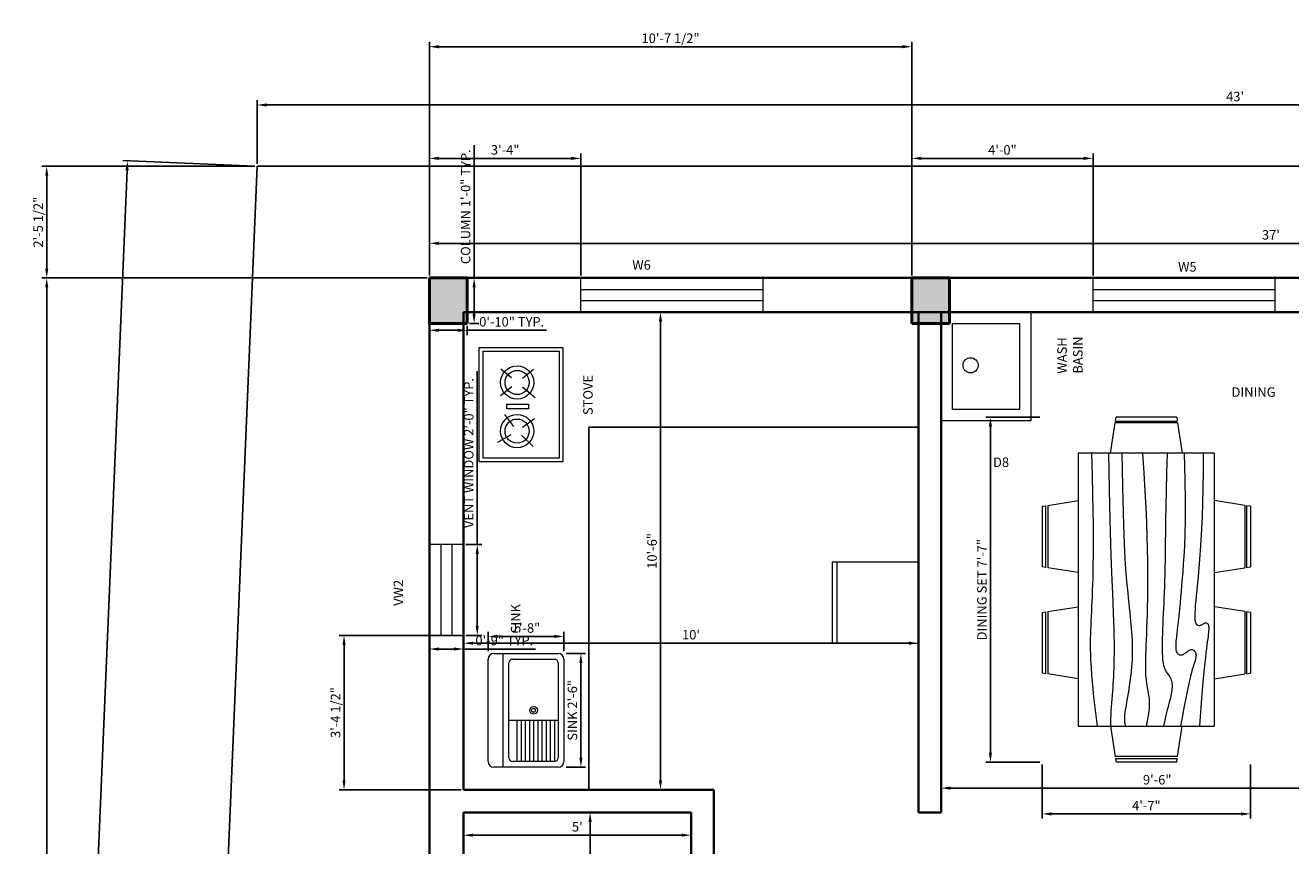
# Model space of a CAD drawing. Units: inches. Extents: x 2470 to 6338, y 1562 to 4199.
# Tile 3 of 5: x 2470 to 2803, y 1985 to 2201. Entities that reach past the tile are written whole.
import ezdxf

# ---------------------------------------------------------------- set-up
doc = ezdxf.new("R2010")
doc.units = ezdxf.units.IN
for name, color, linetype, lineweight in [('A-ANNO-DIMS', 2, 'Continuous', 18), ('A-ANNO-TEXT', 7, 'Continuous', 18), ('A-AREA-IDEN', 7, 'Continuous', 25), ('A-COLS', 1, 'Continuous', 50), ('A-EQPM', 8, 'Continuous', 18), ('A-FLOR-FIXT', 8, 'Continuous', 18), ('A-FLOR-FIXT-PATT', 8, 'Continuous', 13), ('A-FURN', 8, 'Continuous', 18), ('A-FURN-FIXD', 8, 'Continuous', 25), ('A-GLAZ', 4, 'Continuous', 18), ('A-WALL', 7, 'Continuous', 35), ('C-PROP', 3, 'Continuous', 25)]:
    doc.layers.add(name, color=color, linetype=linetype, lineweight=lineweight)
doc.styles.get("Standard").update_dxf_attribs({"font": 'arial.ttf'})
doc.dimstyles.new('ISO-25', dxfattribs={"dimtxt": 2.5, "dimasz": 2.5, "dimexe": 1.25, "dimexo": 0.625, "dimtad": 1, "dimdec": 1, "dimlunit": 3, "dimtxsty": 'Standard', "dimcen": 2.5, "dimadec": 0, "dimazin": 0, "dimtfac": 1, "dimtdec": 1, "dimtmove": 0, "dimatfit": 3, "dimfxl": 1, "dimarcsym": 0})

# ---------------------------------------------------------------- blocks, each defined once
blk = doc.blocks.new('Dining Set - 36 x 72 in.')
for p, q in [((-22, 27.5), (-22.1562, 26.50042)), ((-22, 27.5), (-6, 27.5)), ((-5.8437, 26.49966), (-6, 27.5)), ((6, 27.5), (5.8438, 26.50042)), ((6, 27.5), (22, 27.5)), ((22.1563, 26.49966), (22, 27.5)), ((-22.2343, 26.00059), (-23.4847, 17.99762)), ((-22.2304, 26), (-5.7608, 26)), ((-5.8416, 26.5), (-22.1534, 26.5)), ((-4.5152, 17.99762), (-5.7655, 25.99926)), ((5.7657, 26.00059), (4.5153, 17.99762)), ((5.7696, 26), (22.2392, 26)), ((22.1584, 26.5), (5.8466, 26.5)), ((23.4848, 17.99762), (22.2345, 25.99926)), ((36, 18), (-36, 18)), ((-36, 18), (-36, -18)), ((36, -18), (36, 18)), ((-45.5, 8), (-44.5004, 8.15617)), ((-45.5, 8), (-45.5, -8)), ((-44.5, -8.15843), (-44.5, 8.15338)), ((-44.0006, 8.23428), (-35.9976, 9.48474)), ((-44, 8.23041), (-44, -8.23915)), ((44.0006, 8.23428), (35.9976, 9.48474)), ((44, 8.23041), (44, -8.23915)), ((44.5, -8.15843), (44.5, 8.15338)), ((45.5, 8), (44.5005, 8.15617)), ((45.5, 8), (45.5, -8)), ((-44.4997, -8.15631), (-45.5, -8)), ((-35.9976, -9.48476), (-43.9993, -8.2345)), ((35.9976, -9.48476), (43.9993, -8.2345)), ((44.4997, -8.15631), (45.5, -8)), ((-36, -18), (36, -18)), ((-22.2343, -26.0006), (-23.4847, -17.99762)), ((-4.5152, -17.99762), (-5.7655, -25.99928)), ((5.7657, -26.0006), (4.5153, -17.99762)), ((23.4848, -17.99762), (22.2345, -25.99928)), ((-22.2304, -26), (-5.7608, -26)), ((-22, -27.5), (-22.1562, -26.50044)), ((-5.8416, -26.5), (-22.1534, -26.5)), ((-5.8437, -26.49967), (-6, -27.5)), ((5.7696, -26), (22.2392, -26)), ((6, -27.5), (5.8438, -26.50044)), ((22.1584, -26.5), (5.8466, -26.5)), ((22.1563, -26.49967), (22, -27.5)), ((-22, -27.5), (-6, -27.5)), ((6, -27.5), (22, -27.5))]:
    blk.add_line(p, q)
for points in [[(-36, 15), (-31.1772, 14.97754), (-26.8079, 14.91406), (-22.8538, 14.81543), (-19.276, 14.6875), (-16.0362, 14.53613), (-13.0957, 14.36718), (-10.4159, 14.18652), (-7.9583, 14), (-5.6904, 13.81315), (-3.6035, 13.63021), (-1.6954, 13.45508), (0.0365, 13.29166), (1.5945, 13.14388), (2.9811, 13.01562), (4.1988, 12.9108), (5.25, 12.83333), (6.1393, 12.78613), (6.8802, 12.76823), (7.4883, 12.77767), (7.9792, 12.8125), (8.3685, 12.87077), (8.6719, 12.95052), (8.9049, 13.0498), (9.0833, 13.16666), (9.2205, 13.29899), (9.3216, 13.44401), (9.3895, 13.59879), (9.4271, 13.76041), (9.4373, 13.92594), (9.4232, 14.09245), (9.3875, 14.257), (9.3333, 14.41666), (9.2638, 14.56917), (9.1836, 14.71484), (9.0975, 14.85465), (9.0104, 14.98958), (8.9272, 15.1206), (8.8529, 15.2487), (8.7922, 15.37483), (8.75, 15.5), (8.7305, 15.62467), (8.7344, 15.74739), (8.7617, 15.86621), (8.8125, 15.97916), (8.8867, 16.08431), (8.9844, 16.17968), (9.1055, 16.26334), (9.25, 16.33333), (9.4189, 16.38802), (9.6172, 16.42708), (9.8506, 16.45052), (10.125, 16.45833), (10.4463, 16.45052), (10.8203, 16.42708), (11.2529, 16.38802), (11.75, 16.33333), (12.3184, 16.26318), (12.9694, 16.17838), (13.7151, 16.07991), (14.5677, 15.96875), (15.5395, 15.84586), (16.6426, 15.71224), (17.8893, 15.56884), (19.2917, 15.41666), (20.859, 15.25667), (22.5879, 15.08984), (24.4721, 14.91715), (26.5052, 14.73958), (28.6809, 14.5581), (30.9929, 14.3737), (33.4347, 14.18733), (36, 14)], [(-36, 10), (-28.9766, 10.14274), (-23.1725, 10.20442), (-18.4241, 10.19775), (-14.5677, 10.13541), (-11.4399, 10.03011), (-8.877, 9.89453), (-6.7154, 9.74137), (-4.7917, 9.58333), (-2.9698, 9.43082), (-1.2246, 9.28515), (0.4415, 9.14534), (2.026, 9.01041), (3.5266, 8.87939), (4.9408, 8.7513), (6.266, 8.62516), (7.5, 8.5), (8.6411, 8.37549), (9.6914, 8.2539), (10.6538, 8.13818), (11.5312, 8.03125), (12.3267, 7.93603), (13.043, 7.85547), (13.6831, 7.79248), (14.25, 7.75), (14.7471, 7.7303), (15.1797, 7.73307), (15.5537, 7.75732), (15.875, 7.80208), (16.1494, 7.86637), (16.3828, 7.94922), (16.5811, 8.04964), (16.75, 8.16666), (16.8944, 8.29915), (17.0143, 8.44531), (17.1089, 8.60319), (17.1771, 8.77083), (17.218, 8.94629), (17.2305, 9.1276), (17.2137, 9.31282), (17.1667, 9.5), (17.0895, 9.6875), (16.987, 9.875), (16.8649, 10.0625), (16.7292, 10.25), (16.5856, 10.4375), (16.4401, 10.625), (16.2985, 10.8125), (16.1667, 11), (16.05, 11.18733), (15.9518, 11.3737), (15.8752, 11.5581), (15.8229, 11.73958), (15.798, 11.91715), (15.8034, 12.08984), (15.842, 12.25667), (15.9167, 12.41666), (16.0295, 12.56836), (16.1784, 12.70833), (16.3605, 12.83268), (16.5729, 12.9375), (16.8127, 13.01888), (17.0768, 13.07291), (17.3625, 13.0957), (17.6667, 13.08333), (17.9894, 13.03312), (18.3418, 12.94726), (18.7382, 12.82918), (19.1927, 12.68229), (19.7195, 12.51001), (20.3327, 12.31575), (21.0465, 12.10294), (21.875, 11.875), (22.8357, 11.63354), (23.959, 11.37304), (25.2786, 11.08618), (26.8282, 10.76562), (28.6414, 10.40405), (30.752, 9.99414), (33.1936, 9.52856), (36, 9)], [(-36, 5.5), (-30.7157, 5.3348), (-26.069, 5.20963), (-21.9946, 5.11767), (-18.4271, 5.05208), (-15.3009, 5.00602), (-12.5508, 4.97265), (-10.1112, 4.94515), (-7.9167, 4.91666), (-5.909, 4.88167), (-4.0586, 4.83984), (-2.3429, 4.79215), (-0.7396, 4.73958), (0.7739, 4.6831), (2.22, 4.6237), (3.6213, 4.56233), (5, 4.5), (6.373, 4.43782), (7.7344, 4.3776), (9.0723, 4.32129), (10.375, 4.27083), (11.6309, 4.22819), (12.8281, 4.19531), (13.9551, 4.17415), (15, 4.16666), (15.954, 4.17448), (16.819, 4.19791), (17.6001, 4.23698), (18.3021, 4.29166), (18.9299, 4.36198), (19.4883, 4.44791), (19.9823, 4.54948), (20.4167, 4.66666), (20.7969, 4.79899), (21.1302, 4.94401), (21.4245, 5.09879), (21.6875, 5.26041), (21.9271, 5.42594), (22.1511, 5.59245), (22.3672, 5.757), (22.5834, 5.91666), (22.8065, 6.06868), (23.0404, 6.21093), (23.2879, 6.34147), (23.5521, 6.45833), (23.8358, 6.55957), (24.142, 6.64323), (24.4735, 6.70735), (24.8334, 6.75), (25.2235, 6.76969), (25.642, 6.76692), (26.0858, 6.74267), (26.5521, 6.69791), (27.0379, 6.63362), (27.5404, 6.55078), (28.0565, 6.45036), (28.5834, 6.33333), (29.1242, 6.19987), (29.7071, 6.04687), (30.3661, 5.87044), (31.1354, 5.66666), (32.0493, 5.43164), (33.142, 5.16146), (34.4475, 4.85221), (36, 4.5)], [(-36, -1), (-30.7915, -0.6591), (-26.0195, -0.38216), (-21.6519, -0.16284), (-17.6563, 0.00521), (-14.0005, 0.12833), (-10.6523, 0.21289), (-7.5796, 0.26522), (-4.75, 0.29166), (-2.134, 0.29793), (0.2878, 0.28711), (2.5317, 0.26163), (4.6146, 0.22396), (6.5529, 0.17651), (8.3633, 0.12174), (10.0623, 0.06209), (11.6667, 0), (13.1899, -0.06201), (14.6341, -0.1211), (15.9982, -0.17432), (17.2813, -0.21875), (18.4823, -0.25147), (19.6003, -0.26953), (20.6343, -0.27002), (21.5834, -0.25), (22.4481, -0.20768), (23.2357, -0.14584), (23.9549, -0.06836), (24.6146, 0.02083), (25.2235, 0.11784), (25.7904, 0.21875), (26.3241, 0.31966), (26.8334, 0.41666), (27.3265, 0.50618), (27.8099, 0.58593), (28.2894, 0.65397), (28.7709, 0.70833), (29.2601, 0.74707), (29.763, 0.76823), (30.2855, 0.76985), (30.8334, 0.75), (31.4088, 0.70784), (31.9994, 0.64713), (32.589, 0.57275), (33.1615, 0.48958), (33.7008, 0.4025), (34.1908, 0.3164), (34.6153, 0.23616), (34.9584, 0.16666), (35.2099, 0.11165), (35.3848, 0.07031), (35.504, 0.04069), (35.5886, 0.02083), (35.6594, 0.00879), (35.7377, 0.0026), (35.8442, 0.00032), (36, 0)], [(-36, -6.5), (-27.1843, -6.31267), (-20.084, -6.1263), (-14.469, -5.9419), (-10.1094, -5.76042), (-6.7752, -5.58285), (-4.2363, -5.41016), (-2.2629, -5.24333), (-0.625, -5.08334), (0.8708, -4.93099), (2.2715, -4.78646), (3.5872, -4.64974), (4.8281, -4.52084), (6.0046, -4.39974), (7.127, -4.28646), (8.2053, -4.18099), (9.25, -4.08334), (10.2705, -3.99382), (11.2734, -3.91407), (12.2647, -3.84603), (13.25, -3.79167), (14.2354, -3.75293), (15.2266, -3.73177), (16.2295, -3.73015), (17.25, -3.75), (18.2912, -3.79248), (19.3451, -3.85547), (20.4009, -3.93604), (21.4479, -4.03125), (22.4754, -4.13819), (23.4727, -4.25391), (24.4289, -4.37549), (25.3334, -4.5), (26.1785, -4.62492), (26.9694, -4.74935), (27.7145, -4.87281), (28.4219, -4.99479), (29.1, -5.11483), (29.7572, -5.23242), (30.4016, -5.34709), (31.0417, -5.45834), (31.6837, -5.56437), (32.3262, -5.65821), (32.9658, -5.73153), (33.599, -5.77604), (34.2224, -5.78345), (34.8327, -5.74545), (35.4264, -5.65373), (36, -5.5)], [(-36, -10), (-26.4022, -9.81299), (-18.4675, -9.62891), (-11.9839, -9.45069), (-6.7396, -9.28125), (-2.5226, -9.12354), (0.8789, -8.98047), (3.6769, -8.85498), (6.0833, -8.75), (8.2767, -8.66765), (10.3021, -8.60677), (12.1712, -8.56543), (13.8958, -8.54167), (15.4876, -8.53353), (16.9583, -8.53907), (18.3197, -8.55632), (19.5834, -8.58334), (20.7616, -8.61841), (21.8685, -8.66081), (22.9188, -8.71004), (23.9271, -8.76563), (24.9081, -8.82707), (25.8763, -8.89388), (26.8465, -8.96558), (27.8334, -9.04167), (28.8474, -9.12118), (29.8828, -9.20117), (30.93, -9.27824), (31.9792, -9.34896), (33.0205, -9.40991), (34.0443, -9.45768), (35.0407, -9.48885), (36, -9.5)], [(-36, -14.5), (-30.0881, -14.33513), (-25.0332, -14.21224), (-20.7312, -14.12647), (-17.0781, -14.07292), (-13.97, -14.04671), (-11.3027, -14.04297), (-8.9724, -14.05681), (-6.875, -14.08334), (-4.9224, -14.11833), (-3.0905, -14.16016), (-1.3709, -14.20785), (0.2448, -14.26042), (1.7647, -14.3169), (3.1973, -14.3763), (4.5507, -14.43767), (5.8333, -14.5), (7.0554, -14.5621), (8.235, -14.62175), (9.3922, -14.67652), (10.5469, -14.72396), (11.7192, -14.76164), (12.929, -14.78711), (14.1965, -14.79794), (15.5417, -14.79167), (16.9933, -14.76424), (18.6152, -14.70508), (20.4804, -14.60197), (22.6615, -14.44271), (25.2312, -14.21509), (28.2624, -13.9069), (31.8277, -13.50594), (36, -13)]]:
    blk.add_lwpolyline(points)
blk = doc.blocks.new('Sink-single - 30 in top')
blk.add_line((-15, -3.999996), (15, -3.999996))
for points in [[(-13.5, 0), (13.5, 0)], [(-15, -18.499996), (-15, -1.5)], [(15, -1.5), (15, -18.499996)], [(-13.5, -17.499996), (-13.5, -6.499996)], [(-12.5, -5.499996), (12.5, -5.499996)], [(13.5, -6.499996), (13.5, -17.499996)], [(13.5, -19.999996), (-13.5, -19.999996)], [(12.5, -18.499996), (-12.5, -18.499996)]]:
    blk.add_lwpolyline(points)
for radius in [1, 0.5]:
    blk.add_circle((0, -11.999996), radius)
for centre, radius, start, end in [((-13.5, -1.5), 1.5, 90, 180), ((13.5, -1.5), 1.5, 0, 90), ((-12.5, -6.499996), 1, 90, 180), ((12.5, -6.499996), 1, 0, 90), ((-13.5, -18.499996), 1.5, 180, 270), ((-12.5, -17.499996), 1, 180, 270), ((12.5, -17.499996), 1, 270, 0), ((13.5, -18.499996), 1.5, 270, 0)]:
    blk.add_arc(centre, radius, start, end)
blk = doc.blocks.new('*D7')
at = {"layer": 'A-ANNO-DIMS', "color": 0, "lineweight": -2, "transparency": 16777216}
for p, q in [((2530.1, 2164.02), (2495.24, 2165.49)), ((2496.38, 2162.94), (2472.59, 1598.93)), ((2506.1, 1595.02), (2471.24, 1596.49))]:
    blk.add_line(p, q, dxfattribs=at)
at = {"layer": 'A-ANNO-DIMS', "color": 0, "lineweight": 100, "transparency": 16777216}
for points in [[(2495.96, 2162.95), (2496.8, 2162.92), (2496.48, 2165.43)], [(2472.17, 1598.95), (2473.01, 1598.92), (2472.48, 1596.43)]]:
    blk.add_solid(points, dxfattribs=at)
at = {"layer": 'Defpoints', "color": 0, "lineweight": 100, "transparency": 16777216}
for p in [(2530.72, 2163.99), (2472.48, 1596.43), (2506.72, 1594.99)]:
    blk.add_point(p, dxfattribs=at)
at = {"layer": 'A-ANNO-DIMS', "color": 0, "transparency": 16777216, "insert": (2482.59, 1881.01), "char_height": 2.5, "attachment_point": 5, "rotation": 87.5847}
blk.add_mtext('47\'-5.5"', dxfattribs=at)
blk = doc.blocks.new('*D8')
at = {"layer": 'A-ANNO-DIMS', "color": 0, "lineweight": -2, "transparency": 16777216}
for p, q in [((2530.72, 2164.62), (2530.72, 2181.42)), ((2533.22, 2180.17), (3044.22, 2180.17)), ((3046.72, 2164.62), (3046.72, 2181.42))]:
    blk.add_line(p, q, dxfattribs=at)
at = {"layer": 'A-ANNO-DIMS', "color": 0, "lineweight": 100, "transparency": 16777216}
for points in [[(2533.22, 2180.59), (2533.22, 2179.75), (2530.72, 2180.17)], [(3044.22, 2180.59), (3044.22, 2179.75), (3046.72, 2180.17)]]:
    blk.add_solid(points, dxfattribs=at)
at = {"layer": 'Defpoints', "color": 0, "lineweight": 100, "transparency": 16777216}
for p in [(3046.72, 2180.17), (2530.72, 2163.99), (3046.72, 2163.99)]:
    blk.add_point(p, dxfattribs=at)
at = {"layer": 'A-ANNO-DIMS', "color": 0, "transparency": 16777216, "insert": (2788.72, 2182.07), "char_height": 2.5, "attachment_point": 5}
blk.add_mtext("43'", dxfattribs=at)
blk = doc.blocks.new('*D11')
at = {"layer": 'A-ANNO-DIMS', "color": 0, "lineweight": -2, "transparency": 16777216}
for p, q in [((2576.17, 2135.16), (2576.17, 2144.92)), ((3017.67, 2143.67), (2578.67, 2143.67)), ((3020.17, 2135.16), (3020.17, 2144.92))]:
    blk.add_line(p, q, dxfattribs=at)
at = {"layer": 'A-ANNO-DIMS', "color": 0, "lineweight": 100, "transparency": 16777216}
for points in [[(2578.67, 2144.09), (2578.67, 2143.26), (2576.17, 2143.67)], [(3017.67, 2144.09), (3017.67, 2143.26), (3020.17, 2143.67)]]:
    blk.add_solid(points, dxfattribs=at)
at = {"layer": 'Defpoints', "color": 0, "lineweight": 100, "transparency": 16777216}
for p in [(2576.17, 2143.67), (2576.17, 2134.53), (3020.17, 2134.53)]:
    blk.add_point(p, dxfattribs=at)
at = {"layer": 'A-ANNO-DIMS', "color": 0, "transparency": 16777216, "insert": (2798.17, 2145.58), "char_height": 2.5, "attachment_point": 5}
blk.add_mtext("37'", dxfattribs=at)
blk = doc.blocks.new('*D23')
at = {"layer": 'A-ANNO-DIMS', "color": 0, "lineweight": -2, "transparency": 16777216}
for p, q in [((2615.79, 1993.53), (2619.79, 1993.53)), ((2618.54, 1991.03), (2618.54, 1948.03)), ((2615.79, 1945.53), (2619.79, 1945.53))]:
    blk.add_line(p, q, dxfattribs=at)
at = {"layer": 'A-ANNO-DIMS', "color": 0, "lineweight": 100, "transparency": 16777216}
for points in [[(2618.13, 1991.03), (2618.96, 1991.03), (2618.54, 1993.53)], [(2618.13, 1948.03), (2618.96, 1948.03), (2618.54, 1945.53)]]:
    blk.add_solid(points, dxfattribs=at)
at = {"layer": 'Defpoints', "color": 0, "lineweight": 100, "transparency": 16777216}
for p in [(2615.17, 1993.53), (2615.17, 1945.53), (2618.54, 1945.53)]:
    blk.add_point(p, dxfattribs=at)
at = {"layer": 'A-ANNO-DIMS', "color": 0, "transparency": 16777216, "insert": (2616.67, 1969.53), "char_height": 2.5, "attachment_point": 5, "rotation": 90}
blk.add_mtext("4'", dxfattribs=at)
blk = doc.blocks.new('*D24')
at = {"layer": 'A-ANNO-DIMS', "color": 0, "lineweight": -2, "transparency": 16777216}
for p, q in [((2585.17, 1987.41), (2585.17, 1986.28)), ((2587.67, 1987.53), (2642.67, 1987.53)), ((2645.17, 1988.16), (2645.17, 1988.78))]:
    blk.add_line(p, q, dxfattribs=at)
at = {"layer": 'A-ANNO-DIMS', "color": 0, "lineweight": 100, "transparency": 16777216}
for points in [[(2587.67, 1987.95), (2587.67, 1987.12), (2585.17, 1987.53)], [(2642.67, 1987.95), (2642.67, 1987.12), (2645.17, 1987.53)]]:
    blk.add_solid(points, dxfattribs=at)
at = {"layer": 'Defpoints', "color": 0, "lineweight": 100, "transparency": 16777216}
for p in [(2585.17, 1988.04), (2645.17, 1987.53), (2645.17, 1987.53)]:
    blk.add_point(p, dxfattribs=at)
at = {"layer": 'A-ANNO-DIMS', "color": 0, "transparency": 16777216, "insert": (2615.17, 1989.43), "char_height": 2.5, "attachment_point": 5}
blk.add_mtext("5'", dxfattribs=at)
blk = doc.blocks.new('*D25')
at = {"layer": 'A-ANNO-DIMS', "color": 0, "lineweight": -2, "transparency": 16777216}
for p, q in [((2628.82, 2125.53), (2638.36, 2125.53)), ((2637.11, 2123.03), (2637.11, 2002.03)), ((2628.82, 1999.53), (2638.36, 1999.53))]:
    blk.add_line(p, q, dxfattribs=at)
at = {"layer": 'A-ANNO-DIMS', "color": 0, "lineweight": 100, "transparency": 16777216}
for points in [[(2636.69, 2123.03), (2637.53, 2123.03), (2637.11, 2125.53)], [(2636.69, 2002.03), (2637.53, 2002.03), (2637.11, 1999.53)]]:
    blk.add_solid(points, dxfattribs=at)
at = {"layer": 'Defpoints', "color": 0, "lineweight": 100, "transparency": 16777216}
for p in [(2628.2, 2125.53), (2628.2, 1999.53), (2637.11, 1999.53)]:
    blk.add_point(p, dxfattribs=at)
at = {"layer": 'A-ANNO-DIMS', "color": 0, "transparency": 16777216, "insert": (2635.21, 2062.53), "char_height": 2.5, "attachment_point": 5, "rotation": 90}
blk.add_mtext('10\'-6"', dxfattribs=at)
blk = doc.blocks.new('*D26')
at = {"layer": 'A-ANNO-DIMS', "color": 0, "lineweight": -2, "transparency": 16777216}
for p, q in [((2585.17, 2051.62), (2585.17, 2036.94)), ((2705.17, 2051.62), (2705.17, 2036.94)), ((2587.67, 2038.19), (2702.67, 2038.19))]:
    blk.add_line(p, q, dxfattribs=at)
at = {"layer": 'A-ANNO-DIMS', "color": 0, "lineweight": 100, "transparency": 16777216}
for points in [[(2587.67, 2038.6), (2587.67, 2037.77), (2585.17, 2038.19)], [(2702.67, 2038.6), (2702.67, 2037.77), (2705.17, 2038.19)]]:
    blk.add_solid(points, dxfattribs=at)
at = {"layer": 'Defpoints', "color": 0, "lineweight": 100, "transparency": 16777216}
for p in [(2585.17, 2052.25), (2705.17, 2052.25), (2705.17, 2038.19)]:
    blk.add_point(p, dxfattribs=at)
at = {"layer": 'A-ANNO-DIMS', "color": 0, "transparency": 16777216, "insert": (2645.17, 2040.09), "char_height": 2.5, "attachment_point": 5}
blk.add_mtext("10'", dxfattribs=at)
blk = doc.blocks.new('*D27')
at = {"layer": 'A-ANNO-DIMS', "color": 0, "lineweight": -2, "transparency": 16777216}
for p, q in [((2711.17, 2058.91), (2711.17, 1998.69)), ((2825.17, 2058.91), (2825.17, 1998.69)), ((2713.67, 1999.94), (2822.67, 1999.94))]:
    blk.add_line(p, q, dxfattribs=at)
at = {"layer": 'A-ANNO-DIMS', "color": 0, "lineweight": 100, "transparency": 16777216}
for points in [[(2713.67, 2000.36), (2713.67, 1999.53), (2711.17, 1999.94)], [(2822.67, 2000.36), (2822.67, 1999.53), (2825.17, 1999.94)]]:
    blk.add_solid(points, dxfattribs=at)
at = {"layer": 'Defpoints', "color": 0, "lineweight": 100, "transparency": 16777216}
for p in [(2711.17, 2059.53), (2825.17, 2059.53), (2825.17, 1999.94)]:
    blk.add_point(p, dxfattribs=at)
at = {"layer": 'A-ANNO-DIMS', "color": 0, "transparency": 16777216, "insert": (2768.17, 2001.84), "char_height": 2.5, "attachment_point": 5}
blk.add_mtext('9\'-6"', dxfattribs=at)
blk = doc.blocks.new('WIN-48IN')
for p, q in [((0, 9), (48, 9)), ((0, 0), (0, 9)), ((48, 9), (48, 0)), ((0, 6), (48, 6)), ((48, 3), (0, 3)), ((48, 0), (0, 0))]:
    blk.add_line(p, q)
blk = doc.blocks.new('VENT-WIN-24IN')
for p, q in [((9, 24), (0, 24)), ((0, 24), (0, 0)), ((3, 24), (3, 0)), ((6, 0), (6, 24)), ((9, 0), (9, 24)), ((0, 0), (9, 0))]:
    blk.add_line(p, q)
blk = doc.blocks.new('COL-10X12')
h = blk.add_hatch(color=256)
h.dxf.hatch_style = 1
h.paths.add_polyline_path([(10, 12), (0, 12), (0, 0), (10, 0)])
for p, q in [((10, 12), (0, 12)), ((0, 12), (0, 0)), ((10, 0), (10, 12)), ((0, 0), (10, 0))]:
    blk.add_line(p, q)
blk = doc.blocks.new('*D42')
at = {"layer": 'A-ANNO-DIMS', "color": 0, "lineweight": -2, "transparency": 16777216}
for p, q in [((2588.77, 2064.25), (2588.77, 2109.95)), ((2585.79, 2064.25), (2590.02, 2064.25)), ((2588.77, 2042.75), (2588.77, 2061.75)), ((2585.79, 2040.25), (2590.02, 2040.25))]:
    blk.add_line(p, q, dxfattribs=at)
at = {"layer": 'A-ANNO-DIMS', "color": 0, "lineweight": 100, "transparency": 16777216}
for points in [[(2588.35, 2061.75), (2589.18, 2061.75), (2588.77, 2064.25)], [(2588.35, 2042.75), (2589.18, 2042.75), (2588.77, 2040.25)]]:
    blk.add_solid(points, dxfattribs=at)
at = {"layer": 'Defpoints', "color": 0, "lineweight": 100, "transparency": 16777216}
for p in [(2585.17, 2064.25), (2588.77, 2064.25), (2585.17, 2040.25)]:
    blk.add_point(p, dxfattribs=at)
at = {"layer": 'A-ANNO-DIMS', "color": 0, "transparency": 16777216, "insert": (2586.85, 2088.35), "char_height": 2.5, "attachment_point": 5, "rotation": 90}
blk.add_mtext('VENT WINDOW 2\'-0" TYP.', dxfattribs=at)
blk = doc.blocks.new('*D43')
at = {"layer": 'A-ANNO-DIMS', "color": 0, "lineweight": -2, "transparency": 16777216}
for p, q in [((2576.17, 2039.62), (2576.17, 2035.4)), ((2578.67, 2036.65), (2582.67, 2036.65)), ((2585.17, 2039.62), (2585.17, 2035.4)), ((2585.17, 2036.65), (2604.16, 2036.65))]:
    blk.add_line(p, q, dxfattribs=at)
at = {"layer": 'A-ANNO-DIMS', "color": 0, "lineweight": 100, "transparency": 16777216}
for points in [[(2578.67, 2037.06), (2578.67, 2036.23), (2576.17, 2036.65)], [(2582.67, 2037.06), (2582.67, 2036.23), (2585.17, 2036.65)]]:
    blk.add_solid(points, dxfattribs=at)
at = {"layer": 'Defpoints', "color": 0, "lineweight": 100, "transparency": 16777216}
for p in [(2576.17, 2040.25), (2585.17, 2040.25), (2585.17, 2036.65)]:
    blk.add_point(p, dxfattribs=at)
at = {"layer": 'A-ANNO-DIMS', "color": 0, "transparency": 16777216, "insert": (2595.91, 2038.55), "char_height": 2.5, "attachment_point": 5}
blk.add_mtext('0\'-9" TYP.', dxfattribs=at)
blk = doc.blocks.new('*D44')
at = {"layer": 'A-ANNO-DIMS', "color": 0, "lineweight": -2, "transparency": 16777216}
for p, q in [((2587.94, 2134.53), (2587.94, 2169.6)), ((2586.76, 2134.53), (2589.19, 2134.53)), ((2587.94, 2125.03), (2587.94, 2132.03)), ((2586.76, 2122.53), (2589.19, 2122.53))]:
    blk.add_line(p, q, dxfattribs=at)
at = {"layer": 'A-ANNO-DIMS', "color": 0, "lineweight": 100, "transparency": 16777216}
for points in [[(2587.52, 2132.03), (2588.35, 2132.03), (2587.94, 2134.53)], [(2587.52, 2125.03), (2588.35, 2125.03), (2587.94, 2122.53)]]:
    blk.add_solid(points, dxfattribs=at)
at = {"layer": 'Defpoints', "color": 0, "lineweight": 100, "transparency": 16777216}
for p in [(2586.14, 2134.53), (2587.94, 2134.53), (2586.14, 2122.53)]:
    blk.add_point(p, dxfattribs=at)
at = {"layer": 'A-ANNO-DIMS', "color": 0, "transparency": 16777216, "insert": (2586.02, 2153.32), "char_height": 2.5, "attachment_point": 5, "rotation": 90}
blk.add_mtext('COLUMN 1\'-0" TYP.', dxfattribs=at)
blk = doc.blocks.new('*D45')
at = {"layer": 'A-ANNO-DIMS', "color": 0, "lineweight": -2, "transparency": 16777216}
for p, q in [((2576.14, 2121.91), (2576.14, 2119.48)), ((2578.64, 2120.73), (2583.64, 2120.73)), ((2586.14, 2121.91), (2586.14, 2119.48)), ((2586.14, 2120.73), (2607.07, 2120.73))]:
    blk.add_line(p, q, dxfattribs=at)
at = {"layer": 'A-ANNO-DIMS', "color": 0, "lineweight": 100, "transparency": 16777216}
for points in [[(2578.64, 2121.15), (2578.64, 2120.32), (2576.14, 2120.73)], [(2583.64, 2121.15), (2583.64, 2120.32), (2586.14, 2120.73)]]:
    blk.add_solid(points, dxfattribs=at)
at = {"layer": 'Defpoints', "color": 0, "lineweight": 100, "transparency": 16777216}
for p in [(2576.14, 2122.53), (2586.14, 2122.53), (2586.14, 2120.73)]:
    blk.add_point(p, dxfattribs=at)
at = {"layer": 'A-ANNO-DIMS', "color": 0, "transparency": 16777216, "insert": (2597.85, 2122.64), "char_height": 2.5, "attachment_point": 5}
blk.add_mtext('0\'-10" TYP.', dxfattribs=at)
blk = doc.blocks.new('*D52')
at = {"layer": 'A-ANNO-DIMS', "color": 0, "lineweight": -2, "transparency": 16777216}
for p, q in [((2737.18, 2097.8), (2722.91, 2097.8)), ((2724.16, 2095.3), (2724.16, 2009.3)), ((2737.18, 2006.8), (2722.91, 2006.8))]:
    blk.add_line(p, q, dxfattribs=at)
at = {"layer": 'A-ANNO-DIMS', "color": 0, "lineweight": 100, "transparency": 16777216}
for points in [[(2723.74, 2095.3), (2724.58, 2095.3), (2724.16, 2097.8)], [(2723.74, 2009.3), (2724.58, 2009.3), (2724.16, 2006.8)]]:
    blk.add_solid(points, dxfattribs=at)
at = {"layer": 'Defpoints', "color": 0, "lineweight": 100, "transparency": 16777216}
for p in [(2737.81, 2097.8), (2724.16, 2006.8), (2737.81, 2006.8)]:
    blk.add_point(p, dxfattribs=at)
at = {"layer": 'A-ANNO-DIMS', "color": 0, "transparency": 16777216, "insert": (2722.24, 2052.3), "char_height": 2.5, "attachment_point": 5, "rotation": 90}
blk.add_mtext('DINING SET 7\'-7"', dxfattribs=at)
blk = doc.blocks.new('*D53')
at = {"layer": 'A-ANNO-DIMS', "color": 0, "lineweight": -2, "transparency": 16777216}
for p, q in [((2737.81, 2006.17), (2737.81, 1991.9)), ((2792.81, 2006.17), (2792.81, 1991.9)), ((2740.31, 1993.15), (2790.31, 1993.15))]:
    blk.add_line(p, q, dxfattribs=at)
at = {"layer": 'A-ANNO-DIMS', "color": 0, "lineweight": 100, "transparency": 16777216}
for points in [[(2740.31, 1993.56), (2740.31, 1992.73), (2737.81, 1993.15)], [(2790.31, 1993.56), (2790.31, 1992.73), (2792.81, 1993.15)]]:
    blk.add_solid(points, dxfattribs=at)
at = {"layer": 'Defpoints', "color": 0, "lineweight": 100, "transparency": 16777216}
for p in [(2737.81, 2006.8), (2792.81, 2006.8), (2792.81, 1993.15)]:
    blk.add_point(p, dxfattribs=at)
at = {"layer": 'A-ANNO-DIMS', "color": 0, "transparency": 16777216, "insert": (2765.31, 1995.02), "char_height": 2.5, "attachment_point": 5}
blk.add_mtext('4\'-7"', dxfattribs=at)
blk = doc.blocks.new('*D54')
at = {"layer": 'A-ANNO-DIMS', "color": 0, "lineweight": -2, "transparency": 16777216}
for p, q in [((2612.24, 2035.47), (2617.37, 2035.47)), ((2616.12, 2007.97), (2616.12, 2032.97)), ((2612.24, 2005.47), (2617.37, 2005.47))]:
    blk.add_line(p, q, dxfattribs=at)
at = {"layer": 'A-ANNO-DIMS', "color": 0, "lineweight": 100, "transparency": 16777216}
for points in [[(2615.7, 2032.97), (2616.53, 2032.97), (2616.12, 2035.47)], [(2615.7, 2007.97), (2616.53, 2007.97), (2616.12, 2005.47)]]:
    blk.add_solid(points, dxfattribs=at)
at = {"layer": 'Defpoints', "color": 0, "lineweight": 100, "transparency": 16777216}
for p in [(2611.62, 2035.47), (2616.12, 2035.47), (2611.62, 2005.47)]:
    blk.add_point(p, dxfattribs=at)
at = {"layer": 'A-ANNO-DIMS', "color": 0, "transparency": 16777216, "insert": (2614.2, 2020.47), "char_height": 2.5, "attachment_point": 5, "rotation": 90}
blk.add_mtext('SINK 2\'-6"', dxfattribs=at)
blk = doc.blocks.new('*D55')
at = {"layer": 'A-ANNO-DIMS', "color": 0, "lineweight": -2, "transparency": 16777216}
for p, q in [((2591.62, 2036.1), (2591.62, 2041.22)), ((2609.12, 2039.97), (2594.12, 2039.97)), ((2611.62, 2036.1), (2611.62, 2041.22))]:
    blk.add_line(p, q, dxfattribs=at)
at = {"layer": 'A-ANNO-DIMS', "color": 0, "lineweight": 100, "transparency": 16777216}
for points in [[(2594.12, 2040.39), (2594.12, 2039.56), (2591.62, 2039.97)], [(2609.12, 2040.39), (2609.12, 2039.56), (2611.62, 2039.97)]]:
    blk.add_solid(points, dxfattribs=at)
at = {"layer": 'Defpoints', "color": 0, "lineweight": 100, "transparency": 16777216}
for p in [(2591.62, 2039.97), (2591.62, 2035.47), (2611.62, 2035.47)]:
    blk.add_point(p, dxfattribs=at)
at = {"layer": 'A-ANNO-DIMS', "color": 0, "transparency": 16777216, "insert": (2601.62, 2041.87), "char_height": 2.5, "attachment_point": 5}
blk.add_mtext('1\'-8"', dxfattribs=at)
blk = doc.blocks.new('*D59')
at = {"layer": 'A-ANNO-DIMS', "color": 0, "lineweight": -2, "transparency": 16777216}
for p, q in [((2575.54, 2134.53), (2473.92, 2134.53)), ((2475.17, 1672.03), (2475.17, 2132.03)), ((2527.54, 1669.53), (2473.92, 1669.53))]:
    blk.add_line(p, q, dxfattribs=at)
at = {"layer": 'A-ANNO-DIMS', "color": 0, "lineweight": 100, "transparency": 16777216}
for points in [[(2474.76, 2132.03), (2475.59, 2132.03), (2475.17, 2134.53)], [(2474.76, 1672.03), (2475.59, 1672.03), (2475.17, 1669.53)]]:
    blk.add_solid(points, dxfattribs=at)
at = {"layer": 'Defpoints', "color": 0, "lineweight": 100, "transparency": 16777216}
for p in [(2475.17, 2134.53), (2576.17, 2134.53), (2528.17, 1669.53)]:
    blk.add_point(p, dxfattribs=at)
at = {"layer": 'A-ANNO-DIMS', "color": 0, "transparency": 16777216, "insert": (2473.27, 1902.03), "char_height": 2.5, "attachment_point": 5, "rotation": 90}
blk.add_mtext('38\'-9"', dxfattribs=at)
blk = doc.blocks.new('*D60')
at = {"layer": 'A-ANNO-DIMS', "color": 0, "lineweight": -2, "transparency": 16777216}
for p, q in [((2576.14, 2135.16), (2576.14, 2196.79)), ((2578.64, 2195.54), (2700.91, 2195.54)), ((2703.41, 2135.16), (2703.41, 2196.79))]:
    blk.add_line(p, q, dxfattribs=at)
at = {"layer": 'A-ANNO-DIMS', "color": 0, "lineweight": 100, "transparency": 16777216}
for points in [[(2578.64, 2195.96), (2578.64, 2195.12), (2576.14, 2195.54)], [(2700.91, 2195.96), (2700.91, 2195.12), (2703.41, 2195.54)]]:
    blk.add_solid(points, dxfattribs=at)
at = {"layer": 'Defpoints', "color": 0, "lineweight": 100, "transparency": 16777216}
for p in [(2703.41, 2195.54), (2576.14, 2134.53), (2703.41, 2134.53)]:
    blk.add_point(p, dxfattribs=at)
at = {"layer": 'A-ANNO-DIMS', "color": 0, "transparency": 16777216, "insert": (2639.77, 2197.46), "char_height": 2.5, "attachment_point": 5}
blk.add_mtext('10\'-7 1/2"', dxfattribs=at)
blk = doc.blocks.new('*D67')
at = {"layer": 'A-ANNO-DIMS', "color": 0, "lineweight": -2, "transparency": 16777216}
for p, q in [((2530.1, 2163.99), (2473.92, 2163.99)), ((2475.17, 2137.03), (2475.17, 2161.49)), ((2575.51, 2134.53), (2473.92, 2134.53))]:
    blk.add_line(p, q, dxfattribs=at)
at = {"layer": 'A-ANNO-DIMS', "color": 0, "lineweight": 100, "transparency": 16777216}
for points in [[(2474.76, 2161.49), (2475.59, 2161.49), (2475.17, 2163.99)], [(2474.76, 2137.03), (2475.59, 2137.03), (2475.17, 2134.53)]]:
    blk.add_solid(points, dxfattribs=at)
at = {"layer": 'Defpoints', "color": 0, "lineweight": 100, "transparency": 16777216}
for p in [(2475.17, 2163.99), (2530.72, 2163.99), (2576.14, 2134.53)]:
    blk.add_point(p, dxfattribs=at)
at = {"layer": 'A-ANNO-DIMS', "color": 0, "transparency": 16777216, "insert": (2473.25, 2149.26), "char_height": 2.5, "attachment_point": 5, "rotation": 90}
blk.add_mtext('2\'-5 1/2"', dxfattribs=at)
blk = doc.blocks.new('*D70')
at = {"layer": 'A-ANNO-DIMS', "color": 0, "lineweight": -2, "transparency": 16777216}
for p, q in [((2576.14, 2135.16), (2576.14, 2167.33)), ((2616.12, 2135.16), (2616.12, 2167.33)), ((2578.64, 2166.08), (2613.62, 2166.08))]:
    blk.add_line(p, q, dxfattribs=at)
at = {"layer": 'A-ANNO-DIMS', "color": 0, "lineweight": 100, "transparency": 16777216}
for points in [[(2578.64, 2166.5), (2578.64, 2165.67), (2576.14, 2166.08)], [(2613.62, 2166.5), (2613.62, 2165.67), (2616.12, 2166.08)]]:
    blk.add_solid(points, dxfattribs=at)
at = {"layer": 'Defpoints', "color": 0, "lineweight": 100, "transparency": 16777216}
for p in [(2616.12, 2166.08), (2576.14, 2134.53), (2616.12, 2134.53)]:
    blk.add_point(p, dxfattribs=at)
at = {"layer": 'A-ANNO-DIMS', "color": 0, "transparency": 16777216, "insert": (2596.13, 2167.99), "char_height": 2.5, "attachment_point": 5}
blk.add_mtext('3\'-4"', dxfattribs=at)
blk = doc.blocks.new('*D71')
at = {"layer": 'A-ANNO-DIMS', "color": 0, "lineweight": -2, "transparency": 16777216}
for p, q in [((2703.41, 2135.16), (2703.41, 2167.33)), ((2751.24, 2135.16), (2751.24, 2167.33)), ((2705.91, 2166.08), (2748.74, 2166.08))]:
    blk.add_line(p, q, dxfattribs=at)
at = {"layer": 'A-ANNO-DIMS', "color": 0, "lineweight": 100, "transparency": 16777216}
for points in [[(2705.91, 2166.5), (2705.91, 2165.67), (2703.41, 2166.08)], [(2748.74, 2166.5), (2748.74, 2165.67), (2751.24, 2166.08)]]:
    blk.add_solid(points, dxfattribs=at)
at = {"layer": 'Defpoints', "color": 0, "lineweight": 100, "transparency": 16777216}
for p in [(2751.24, 2166.08), (2703.41, 2134.53), (2751.24, 2134.53)]:
    blk.add_point(p, dxfattribs=at)
at = {"layer": 'A-ANNO-DIMS', "color": 0, "transparency": 16777216, "insert": (2727.33, 2167.99), "char_height": 2.5, "attachment_point": 5}
blk.add_mtext('4\'-0"', dxfattribs=at)
blk = doc.blocks.new('*D76')
at = {"layer": 'A-ANNO-DIMS', "color": 0, "lineweight": -2, "transparency": 16777216}
for p, q in [((2584.54, 2040.25), (2552.37, 2040.25)), ((2553.62, 2002.03), (2553.62, 2037.75)), ((2584.54, 1999.53), (2552.37, 1999.53))]:
    blk.add_line(p, q, dxfattribs=at)
at = {"layer": 'A-ANNO-DIMS', "color": 0, "lineweight": 100, "transparency": 16777216}
for points in [[(2553.2, 2037.75), (2554.03, 2037.75), (2553.62, 2040.25)], [(2553.2, 2002.03), (2554.03, 2002.03), (2553.62, 1999.53)]]:
    blk.add_solid(points, dxfattribs=at)
at = {"layer": 'Defpoints', "color": 0, "lineweight": 100, "transparency": 16777216}
for p in [(2553.62, 2040.25), (2585.17, 2040.25), (2585.17, 1999.53)]:
    blk.add_point(p, dxfattribs=at)
at = {"layer": 'A-ANNO-DIMS', "color": 0, "transparency": 16777216, "insert": (2551.7, 2019.89), "char_height": 2.5, "attachment_point": 5, "rotation": 90}
blk.add_mtext('3\'-4 1/2"', dxfattribs=at)

msp = doc.modelspace()

# ---------------------------------------------------------------- hatches: boundary and pattern name
at = {"layer": 'A-FLOR-FIXT-PATT'}
h = msp.add_hatch(dxfattribs=at)
h.set_pattern_fill('ANSI31', color=256, scale=0.3464567, angle=45, style=0)
h.paths.add_polyline_path([(2598.22, 2006.97), (2609.22, 2006.97), (2609.22, 2017.9), (2598.22, 2017.9)])

# ---------------------------------------------------------------- linework, layer by layer
at = {"layer": 'A-EQPM'}
for p, q in [((2597.79, 2108.21), (2595.02, 2110.5)), ((2600.67, 2108.07), (2603.62, 2110.45)), ((2597.85, 2105.8), (2594.91, 2103.43)), ((2600.71, 2105.79), (2604.07, 2103.01)), ((2598.41, 2095.35), (2596.07, 2098.55)), ((2600.67, 2095.13), (2603.89, 2097.48)), ((2597.6, 2093.17), (2594.07, 2091.16)), ((2600.41, 2093.05), (2603.51, 2090.04)), ((2683.68, 2059.53), (2683.68, 2038.19))]:
    msp.add_line(p, q, dxfattribs=at)
for points in [[(2589.31, 2116.18), (2611.37, 2116.18), (2611.37, 2086.02), (2589.31, 2086.02)], [(2590.31, 2115.18), (2610.37, 2115.18), (2610.37, 2087.02), (2590.31, 2087.02)], [(2596.53, 2101.21), (2602.29, 2101.21), (2602.29, 2099.98), (2596.53, 2099.98)], [(2705.17, 2059.53), (2682.39, 2059.53), (2682.39, 2038.19), (2705.17, 2038.19)]]:
    msp.add_lwpolyline(points, close=True, dxfattribs=at)
for centre, radius in [((2599.29, 2106.96), 4.39), ((2599.29, 2106.96), 3.19), ((2599.29, 2094.13), 4.39), ((2599.29, 2094.13), 3.19)]:
    msp.add_circle(centre, radius, dxfattribs=at)
at = {"layer": 'A-FLOR-FIXT'}
msp.add_line((2597.12, 2017.9), (2610.12, 2017.9), dxfattribs=at)
for points in [[(2711.17, 2125.53), (2734.83, 2125.53), (2734.83, 2096.81), (2711.17, 2096.81)], [(2714.17, 2122.53), (2731.83, 2122.53), (2731.83, 2099.81), (2714.17, 2099.81)]]:
    msp.add_lwpolyline(points, close=True, dxfattribs=at)
msp.add_circle((2718.93, 2111.49), 2, dxfattribs=at)
at = {"layer": 'A-FURN-FIXD'}
for p, q in [((2618.17, 1999.53), (2618.17, 2095.21)), ((2618.17, 2095.21), (2705.17, 2095.21))]:
    msp.add_line(p, q, dxfattribs=at)
at = {"layer": 'A-WALL'}
for p, q in [((2576.17, 2134.53), (3020.17, 2134.53)), ((2576.17, 1763.15), (2576.17, 2134.53)), ((2585.17, 2125.53), (3011.17, 2125.53)), ((2585.17, 1999.53), (2585.17, 2125.53)), ((2705.17, 1993.53), (2705.17, 2125.53)), ((2711.17, 1993.53), (2711.17, 2125.53)), ((2585.17, 1999.53), (2651.17, 1999.53)), ((2651.17, 1981.53), (2651.17, 1999.53)), ((2585.17, 1993.53), (2645.17, 1993.53)), ((2585.17, 1945.53), (2585.17, 1993.53)), ((2645.17, 1981.53), (2645.17, 1993.53)), ((2705.17, 1993.53), (2711.17, 1993.53))]:
    msp.add_line(p, q, dxfattribs=at)
at = {"layer": 'C-PROP'}
for q in [(2506.72, 1594.99), (3046.72, 2163.99)]:
    msp.add_line((2530.72, 2163.99), q, dxfattribs=at)

# ---------------------------------------------------------------- block references
at = {"layer": 'A-COLS'}
for p in [(2576.14, 2122.53), (2703.41, 2122.53)]:
    msp.add_blockref('COL-10X12', p, dxfattribs=at)
at = {"layer": 'A-FLOR-FIXT', "rotation": 90}
msp.add_blockref('Sink-single - 30 in top', (2591.62, 2020.47), dxfattribs=at)
at = {"layer": 'A-FURN', "rotation": 270}
msp.add_blockref('Dining Set - 36 x 72 in.', (2765.31, 2052.3), dxfattribs=at)
at = {"layer": 'A-GLAZ'}
for name, p in [('WIN-48IN', (2616.12, 2125.53)), ('WIN-48IN', (2751.24, 2125.53)), ('VENT-WIN-24IN', (2576.17, 2040.25))]:
    msp.add_blockref(name, p, dxfattribs=at)

# ---------------------------------------------------------------- texts
at = {"layer": 'A-ANNO-TEXT', "char_height": 2.5, "attachment_point": 1}
for s, width, insert in [('W6', 15.7571, (2629.68, 2139.21)), ('W5', 13.698, (2773.68, 2138.72)), ('D8', 6.2696, (2724.85, 2087.16))]:
    msp.add_mtext_dynamic_manual_height_columns(s, width=width, gutter_width=12.5, heights=[0], dxfattribs=dict(at, insert=insert))
at = {"layer": 'A-ANNO-TEXT', "char_height": 2.5, "attachment_point": 1, "rotation": 90}
for s, width, insert in [('WASH \\PBASIN', 16.8458, (2741.81, 2109.29)), ('STOVE', 17.7623, (2616.73, 2098.37)), ('VW2', 16.2026, (2566.72, 2048.05)), ('SINK', 11.7415, (2597.65, 2040.8))]:
    msp.add_mtext_dynamic_manual_height_columns(s, width=width, gutter_width=12.5, heights=[0], dxfattribs=dict(at, insert=insert))
at = {"layer": 'A-AREA-IDEN', "insert": (2787.77, 2105.68), "char_height": 2.5, "attachment_point": 1}
msp.add_mtext_dynamic_manual_height_columns('DINING', width=24.6621, gutter_width=12.5, heights=[0], dxfattribs=at)

# ---------------------------------------------------------------- dimensions: what is measured, and where the dimension line sits
at = {"layer": 'A-ANNO-DIMS'}
for base, p1, p2, override, picture, middle in [((2703.41, 2195.54), (2576.14, 2134.53), (2703.41, 2134.53), {"dimdec": 1, "dimlfac": 1, "dimrnd": 0, "dimzin": 1, "dimdsep": 46, "dimlunit": 4, "dimfrac": 2}, '*D60', (2639.77, 2197.46)), ((3046.72, 2180.17), (2530.72, 2163.99), (3046.72, 2163.99), {"dimclrd": 0, "dimclre": 0, "dimclrt": 0}, '*D8', (2788.72, 2182.07)), ((2616.12, 2166.08), (2576.14, 2134.53), (2616.12, 2134.53), {"dimdec": 1, "dimlfac": 1, "dimrnd": 0, "dimzin": 1, "dimdsep": 46, "dimlunit": 4, "dimfrac": 2}, '*D70', (2596.13, 2167.99)), ((2576.17, 2143.67), (3020.17, 2134.53), (2576.17, 2134.53), {"dimclrd": 0, "dimclre": 0, "dimclrt": 0}, '*D11', (2798.17, 2145.58)), ((2825.17, 1999.94), (2711.17, 2059.53), (2825.17, 2059.53), {"dimclrd": 0, "dimclre": 0, "dimclrt": 0}, '*D27', (2768.17, 2001.84)), ((2705.17, 2038.19), (2585.17, 2052.25), (2705.17, 2052.25), {"dimclrd": 0, "dimclre": 0, "dimclrt": 0}, '*D26', (2645.17, 2040.09)), ((2792.81, 1993.15), (2737.81, 2006.8), (2792.81, 2006.8), {"dimdec": 1, "dimlfac": 1, "dimrnd": 0, "dimzin": 1, "dimdsep": 46, "dimlunit": 4, "dimfrac": 2}, '*D53', (2765.31, 1995.02)), ((2645.17, 1987.53), (2585.17, 1988.04), (2645.17, 1987.53), {"dimclrd": 0, "dimclre": 0, "dimclrt": 0}, '*D24', (2615.17, 1989.43))]:
    dim = msp.add_linear_dim(base=base, p1=p1, p2=p2, dimstyle='ISO-25', override=override, dxfattribs=at)
    dim.commit()
    dim.dimension.update_dxf_attribs({"geometry": picture, "text_midpoint": middle})
for base, p1, p2, angle, text, picture, middle in [((2587.94, 2134.53), (2586.14, 2122.53), (2586.14, 2134.53), 90, 'COLUMN <> TYP.', '*D44', (2586.02, 2153.32)), ((2588.77, 2064.25), (2585.17, 2040.25), (2585.17, 2064.25), 90, 'VENT WINDOW <> TYP.', '*D42', (2586.85, 2088.35)), ((2724.16, 2006.8), (2737.81, 2097.8), (2737.81, 2006.8), 270, 'DINING SET <>', '*D52', (2722.24, 2052.3)), ((2616.12, 2035.47), (2611.62, 2005.47), (2611.62, 2035.47), 90, 'SINK <>', '*D54', (2614.2, 2020.47))]:
    dim = msp.add_linear_dim(base=base, p1=p1, p2=p2, angle=angle, text=text, dimstyle='ISO-25', override={"dimdec": 1, "dimlfac": 1, "dimrnd": 0, "dimzin": 1, "dimdsep": 46, "dimlunit": 4, "dimfrac": 2}, dxfattribs=at)
    dim.commit()
    dim.dimension.update_dxf_attribs({"geometry": picture, "text_midpoint": middle})
for base, p1, p2, angle, override, picture, middle in [((2751.24, 2166.08), (2703.41, 2134.53), (2751.24, 2134.53), 0, {"dimdec": 1, "dimlfac": 1, "dimrnd": 0, "dimzin": 1, "dimdsep": 46, "dimlunit": 4, "dimfrac": 2}, '*D71', (2727.33, 2167.99)), ((2475.17, 2163.99), (2576.14, 2134.53), (2530.72, 2163.99), 90, {"dimdec": 1, "dimlfac": 1, "dimrnd": 0, "dimzin": 1, "dimdsep": 46, "dimlunit": 4, "dimfrac": 2}, '*D67', (2473.25, 2149.26)), ((2475.17, 2134.53), (2528.17, 1669.53), (2576.17, 2134.53), 90, {"dimdec": 1, "dimlfac": 1, "dimrnd": 0, "dimzin": 1, "dimdsep": 46, "dimlunit": 4, "dimfrac": 2}, '*D59', (2473.27, 1902.03)), ((2637.11, 1999.53), (2628.2, 2125.53), (2628.2, 1999.53), 90, {"dimclrd": 0, "dimclre": 0, "dimclrt": 0}, '*D25', (2635.21, 2062.53)), ((2591.62, 2039.97), (2611.62, 2035.47), (2591.62, 2035.47), 180, {"dimdec": 1, "dimlfac": 1, "dimrnd": 0, "dimzin": 1, "dimdsep": 46, "dimlunit": 4, "dimfrac": 2}, '*D55', (2601.62, 2041.87)), ((2553.62, 2040.25), (2585.17, 1999.53), (2585.17, 2040.25), 90, {"dimdec": 1, "dimlfac": 1, "dimrnd": 0, "dimzin": 1, "dimdsep": 46, "dimlunit": 4, "dimfrac": 2}, '*D76', (2551.7, 2019.89)), ((2618.54, 1945.53), (2615.17, 1993.53), (2615.17, 1945.53), 90, {"dimclrd": 0, "dimclre": 0, "dimclrt": 0}, '*D23', (2616.67, 1969.53))]:
    dim = msp.add_linear_dim(base=base, p1=p1, p2=p2, angle=angle, dimstyle='ISO-25', override=override, dxfattribs=at)
    dim.commit()
    dim.dimension.update_dxf_attribs({"geometry": picture, "text_midpoint": middle})
dim = msp.add_aligned_dim(p1=(2530.72, 2163.99), p2=(2506.72, 1594.99), distance=-34.27, dimstyle='ISO-25', override={"dimclrd": 0, "dimclre": 0, "dimclrt": 0}, dxfattribs=at)
dim.commit()
dim.dimension.update_dxf_attribs({"geometry": '*D7', "text_midpoint": (2482.59, 1881.01)})
for base, p1, p2, picture, middle in [((2586.14, 2120.73), (2576.14, 2122.53), (2586.14, 2122.53), '*D45', (2597.85, 2122.64)), ((2585.17, 2036.65), (2576.17, 2040.25), (2585.17, 2040.25), '*D43', (2595.91, 2038.55))]:
    dim = msp.add_linear_dim(base=base, p1=p1, p2=p2, text='<> TYP.', dimstyle='ISO-25', override={"dimdec": 1, "dimlfac": 1, "dimrnd": 0, "dimzin": 1, "dimdsep": 46, "dimlunit": 4, "dimfrac": 2}, dxfattribs=at)
    dim.commit()
    dim.dimension.update_dxf_attribs({"geometry": picture, "text_midpoint": middle})

doc.saveas('drawing.dxf')
